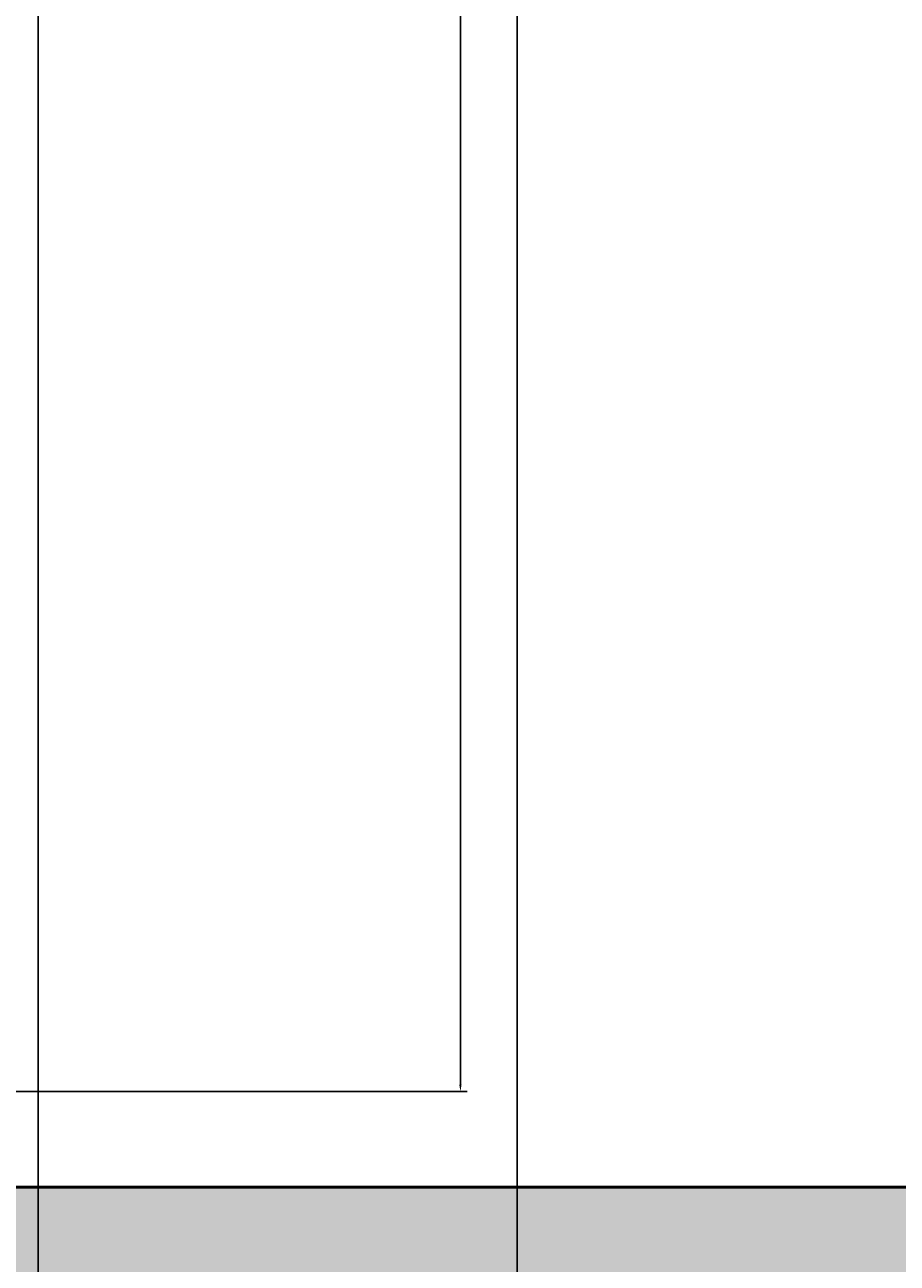
# Model space of a CAD drawing. Units: inches. Extents: x 2231 to 2461, y 2045 to 2455.
# Tile 46 of 95: x 2348 to 2371, y 2185 to 2217. Entities that reach past the tile are written whole.
import ezdxf

# ---------------------------------------------------------------- set-up
doc = ezdxf.new("R2010")
doc.units = ezdxf.units.IN
doc.layers.add('A-ANNO-DIMS', color=2, linetype='Continuous', lineweight=18)
doc.layers.add('A-WALL', color=7, linetype='Continuous', lineweight=50)
doc.layers.add('A-WALL-PATT', color=18, linetype='Continuous', lineweight=13, true_color=0x000000)
doc.styles.get("Standard").update_dxf_attribs({"font": 'arial.ttf'})
doc.dimstyles.get("Standard").update_dxf_attribs({"dimtxt": 0.18, "dimasz": 0.18, "dimexe": 0.18, "dimexo": 0.0625, "dimgap": 0.09, "dimtad": 0, "dimtih": 1, "dimtoh": 1, "dimdec": 4, "dimzin": 0, "dimdsep": 46, "dimtxsty": 'Standard', "dimcen": 0.09, "dimadec": 0, "dimazin": 0, "dimtfac": 1, "dimtdec": 4, "dimtofl": 0, "dimtmove": 0, "dimatfit": 3, "dimfxl": 1, "dimtolj": 1, "dimtzin": 0, "dimarcsym": 0})

# ---------------------------------------------------------------- blocks, each defined once
blk = doc.blocks.new('*D52')
at = {"layer": 'A-ANNO-DIMS', "color": 0, "lineweight": -2, "transparency": 16777216}
for p, q in [((2330.794, 2306.77), (2330.794, 2044.803)), ((2360.794, 2306.77), (2360.794, 2044.803)), ((2330.974, 2044.983), (2345.575, 2044.983)), ((2360.614, 2044.983), (2346.012, 2044.983))]:
    blk.add_line(p, q, dxfattribs=at)
at = {"layer": 'A-ANNO-DIMS', "color": 0, "transparency": 16777216}
for points in [[(2330.974, 2045.013), (2330.974, 2044.953), (2330.794, 2044.983)], [(2360.614, 2045.013), (2360.614, 2044.953), (2360.794, 2044.983)]]:
    blk.add_solid(points, dxfattribs=at)
at = {"layer": 'Defpoints', "color": 0, "transparency": 16777216}
for p in [(2330.794, 2306.833), (2360.794, 2306.833), (2360.794, 2044.983)]:
    blk.add_point(p, dxfattribs=at)
at = {"layer": 'A-ANNO-DIMS', "color": 0, "transparency": 16777216, "insert": (2345.794, 2044.983), "char_height": 0.18, "attachment_point": 5}
blk.add_mtext('\\A1;30', dxfattribs=at)
blk = doc.blocks.new('*D64')
at = {"layer": 'A-ANNO-DIMS', "color": 0, "lineweight": -2, "transparency": 16777216}
for p, q in [((2340.73, 2261.358), (2359.48, 2261.358)), ((2359.3, 2261.178), (2359.3, 2225.535)), ((2359.3, 2189.528), (2359.3, 2225.171)), ((2340.73, 2189.348), (2359.48, 2189.348))]:
    blk.add_line(p, q, dxfattribs=at)
at = {"layer": 'A-ANNO-DIMS', "color": 0, "transparency": 16777216}
for points in [[(2359.27, 2261.178), (2359.33, 2261.178), (2359.3, 2261.358)], [(2359.27, 2189.528), (2359.33, 2189.528), (2359.3, 2189.348)]]:
    blk.add_solid(points, dxfattribs=at)
at = {"layer": 'Defpoints', "color": 0, "transparency": 16777216}
for p in [(2340.667, 2261.358), (2340.667, 2189.348), (2359.3, 2189.348)]:
    blk.add_point(p, dxfattribs=at)
at = {"layer": 'A-ANNO-DIMS', "color": 0, "transparency": 16777216, "insert": (2359.3, 2225.353), "char_height": 0.18, "attachment_point": 5}
blk.add_mtext('\\A1;72.01', dxfattribs=at)
blk = doc.blocks.new('*D66')
at = {"layer": 'A-ANNO-DIMS', "color": 0, "lineweight": -2, "transparency": 16777216}
for p, q in [((2348.189, 2096.895), (2348.189, 2454.645)), ((2408.794, 2096.895), (2408.794, 2454.645)), ((2348.369, 2454.465), (2378.167, 2454.465)), ((2408.614, 2454.465), (2378.815, 2454.465))]:
    blk.add_line(p, q, dxfattribs=at)
at = {"layer": 'A-ANNO-DIMS', "color": 0, "transparency": 16777216}
for points in [[(2348.369, 2454.495), (2348.369, 2454.435), (2348.189, 2454.465)], [(2408.614, 2454.495), (2408.614, 2454.435), (2408.794, 2454.465)]]:
    blk.add_solid(points, dxfattribs=at)
at = {"layer": 'Defpoints', "color": 0, "transparency": 16777216}
for p in [(2408.794, 2454.465), (2348.189, 2096.833), (2408.794, 2096.833)]:
    blk.add_point(p, dxfattribs=at)
at = {"layer": 'A-ANNO-DIMS', "color": 0, "transparency": 16777216, "insert": (2378.491, 2454.465), "char_height": 0.18, "attachment_point": 5}
blk.add_mtext('\\A1;60.6', dxfattribs=at)
blk = doc.blocks.new('*D69')
at = {"layer": 'A-ANNO-DIMS', "color": 0, "lineweight": -2, "transparency": 16777216}
for p, q in [((2340.667, 2189.285), (2340.667, 2044.803)), ((2394.794, 2186.77), (2394.794, 2044.803)), ((2340.847, 2044.983), (2367.337, 2044.983)), ((2394.614, 2044.983), (2368.124, 2044.983))]:
    blk.add_line(p, q, dxfattribs=at)
at = {"layer": 'A-ANNO-DIMS', "color": 0, "transparency": 16777216}
for points in [[(2340.847, 2045.013), (2340.847, 2044.953), (2340.667, 2044.983)], [(2394.614, 2045.013), (2394.614, 2044.953), (2394.794, 2044.983)]]:
    blk.add_solid(points, dxfattribs=at)
at = {"layer": 'Defpoints', "color": 0, "transparency": 16777216}
for p in [(2340.667, 2189.348), (2394.794, 2186.833), (2394.794, 2044.983)]:
    blk.add_point(p, dxfattribs=at)
at = {"layer": 'A-ANNO-DIMS', "color": 0, "transparency": 16777216, "insert": (2367.73, 2044.983), "char_height": 0.18, "attachment_point": 5}
blk.add_mtext('\\A1;54.13', dxfattribs=at)

msp = doc.modelspace()

# ---------------------------------------------------------------- hatches: boundary and pattern name
at = {"layer": 'A-WALL-PATT'}
h = msp.add_hatch(color=256, dxfattribs=at)
h.dxf.hatch_style = 1
h.paths.add_polyline_path([(2441.7935, 2269.1535), (2432.7935, 2269.1535), (2432.7935, 2186.8328), (2396.7935, 2186.8328), (2396.7935, 2286.8328), (2394.7935, 2286.8328), (2394.7935, 2186.8328), (2334.7935, 2186.8328), (2334.7935, 2182.8328), (2432.7935, 2182.8328), (2432.7935, 2072.8328), (2416.6639, 2072.8328), (2416.6639, 2063.8328), (2441.7935, 2063.8328)])
h.paths.add_polyline_path([(2368.6639, 2072.8328), (2367.04, 2072.8328), (2330.7942, 2072.8328), (2330.7397, 2063.8328), (2368.6639, 2063.8328)])
h.paths.add_polyline_path([(2300.7392, 2068.3328), (2300.7392, 2072.8328), (2298.7935, 2072.8328), (2294.7935, 2072.8328), (2258.7935, 2072.8328), (2258.7935, 2120.8328), (2294.7935, 2120.8328), (2298.7935, 2120.8328), (2298.7935, 2128.8328), (2294.7935, 2128.8328), (2294.7935, 2124.8328), (2258.7935, 2124.8328), (2258.7935, 2182.8328), (2294.7935, 2182.8328), (2294.7935, 2174.8328), (2298.7935, 2174.8328), (2298.7935, 2182.8328), (2304.7935, 2182.8328), (2304.7935, 2186.8328), (2258.7935, 2186.8328), (2258.7935, 2221.999), (2249.7935, 2221.999), (2249.7935, 2063.8328), (2300.7392, 2063.8328)])
h.paths.add_polyline_path([(2391.9338, 2435.8328), (2333.82, 2435.8328), (2333.82, 2426.8328), (2368.7935, 2426.8328), (2368.7935, 2374.9508), (2368.7935, 2370.8328), (2372.3935, 2370.8328), (2372.7935, 2370.8328), (2372.7935, 2426.8328), (2391.9338, 2426.8328)])
h.paths.add_polyline_path([(2441.7935, 2435.8328), (2415.9338, 2435.8328), (2415.9338, 2426.8328), (2432.7935, 2426.8328), (2432.7935, 2334.8328), (2372.7935, 2334.8328), (2372.7935, 2346.8328), (2368.7935, 2346.8328), (2368.7935, 2306.8328), (2360.7935, 2306.8328), (2360.7935, 2302.8328), (2368.7935, 2302.8328), (2372.7935, 2302.8328), (2372.7935, 2330.8328), (2432.7935, 2330.8328), (2432.7935, 2317.1535), (2441.7935, 2317.1535)])
h.paths.add_polyline_path([(2285.82, 2435.8328), (2249.7935, 2435.8328), (2249.7935, 2269.999), (2258.7935, 2269.999), (2258.7935, 2302.8328), (2318.8168, 2302.8328), (2330.7935, 2302.8328), (2330.7935, 2306.8328), (2258.7935, 2306.8328), (2258.7935, 2426.8328), (2285.82, 2426.8328)])

# ---------------------------------------------------------------- linework, layer by layer
at = {"layer": 'A-WALL'}
msp.add_line((2334.7935, 2186.8328), (2394.7935, 2186.8328), dxfattribs=at)

# ---------------------------------------------------------------- dimensions: what is measured, and where the dimension line sits
at = {"layer": 'A-ANNO-DIMS'}
for base, p1, p2, override, picture, middle in [((2408.7935, 2454.4653), (2348.1888, 2096.8328), (2408.7935, 2096.8328), {"dimdec": 1, "dimlfac": 1, "dimrnd": 0, "dimzin": 0, "dimdsep": 46, "dimlunit": 2}, '*D66', (2378.4912, 2454.4653)), ((2360.7935, 2044.9825), (2330.7935, 2306.8328), (2360.7935, 2306.8328), {"dimdec": 0, "dimlfac": 1, "dimrnd": 0, "dimzin": 0, "dimdsep": 46, "dimlunit": 2}, '*D52', (2345.7935, 2044.9825)), ((2394.7935, 2044.9825), (2340.6673, 2189.3477), (2394.7935, 2186.8328), {"dimdec": 2, "dimlfac": 1, "dimrnd": 0, "dimzin": 0, "dimdsep": 46, "dimlunit": 2}, '*D69', (2367.7304, 2044.9825))]:
    dim = msp.add_linear_dim(base=base, p1=p1, p2=p2, dimstyle='Standard', override=override, dxfattribs=at)
    dim.commit()
    dim.dimension.update_dxf_attribs({"geometry": picture, "text_midpoint": middle})
dim = msp.add_linear_dim(base=(2359.2998, 2189.3477), p1=(2340.6673, 2261.3584), p2=(2340.6673, 2189.3477), angle=270, dimstyle='Standard', override={"dimdec": 2, "dimlfac": 1, "dimrnd": 0, "dimzin": 0, "dimdsep": 46, "dimlunit": 2}, dxfattribs=at)
dim.commit()
dim.dimension.update_dxf_attribs({"geometry": '*D64', "text_midpoint": (2359.2998, 2225.353)})

doc.saveas('drawing.dxf')
